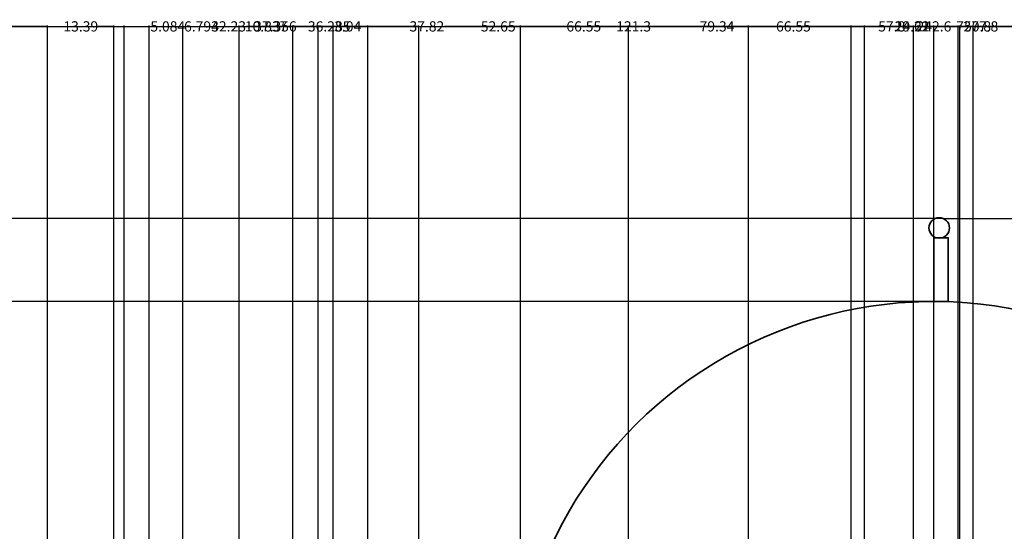
# Model space of a CAD drawing. Units: inches. Extents: x 14 to 859, y 52 to 711.
# Tile 8 of 11: x 244 to 442, y 608 to 711. Entities that reach past the tile are written whole.
import ezdxf

# ---------------------------------------------------------------- set-up
doc = ezdxf.new("R2010")
doc.units = ezdxf.units.IN
doc.header["$MEASUREMENT"] = 0
doc.layers.add('A-ANNO-DIMS', color=2, linetype='Continuous', lineweight=18)
doc.layers.add('A-ROOF', color=7, linetype='Continuous', lineweight=35)
doc.styles.get("Standard").update_dxf_attribs({"font": 'arial.ttf'})
doc.dimstyles.get("Standard").update_dxf_attribs({"dimtxt": 2.0625, "dimasz": 0.18, "dimexe": 0.18, "dimexo": 0.0625, "dimgap": 0.09, "dimtad": 0, "dimtih": 1, "dimtoh": 1, "dimdec": 4, "dimzin": 0, "dimdsep": 46, "dimlunit": 4, "dimtxsty": 'Standard', "dimcen": 0.09, "dimadec": 0, "dimazin": 0, "dimtfac": 1, "dimtdec": 4, "dimtofl": 0, "dimtmove": 0, "dimatfit": 3, "dimfxl": 1, "dimtolj": 1, "dimtzin": 0, "dimarcsym": 0})

# ---------------------------------------------------------------- blocks, each defined once
blk = doc.blocks.new('*D13')
at = {"layer": 'A-ANNO-DIMS', "color": 0, "lineweight": -2, "transparency": 16777216}
for p, q in [((60.78, 339.73), (60.78, 709.71)), ((811.55, 339.73), (811.55, 709.71)), ((60.96, 709.53), (432.6, 709.53)), ((811.37, 709.53), (439.73, 709.53))]:
    blk.add_line(p, q, dxfattribs=at)
at = {"layer": 'A-ANNO-DIMS', "color": 0, "transparency": 16777216}
for points in [[(60.96, 709.56), (60.96, 709.5), (60.78, 709.53)], [(811.37, 709.56), (811.37, 709.5), (811.55, 709.53)]]:
    blk.add_solid(points, dxfattribs=at)
at = {"layer": 'Defpoints', "color": 0, "transparency": 16777216}
for p in [(811.55, 709.53), (60.78, 339.66), (811.55, 339.66)]:
    blk.add_point(p, dxfattribs=at)
at = {"layer": 'A-ANNO-DIMS', "color": 0, "transparency": 16777216, "insert": (436.17, 709.53), "char_height": 2.062, "attachment_point": 5}
blk.add_mtext('\\A1;750.8', dxfattribs=at)
blk = doc.blocks.new('*D16')
at = {"layer": 'A-ANNO-DIMS', "color": 0, "lineweight": -2, "transparency": 16777216}
for p, q in [((429.96, 670.76), (17.7, 670.76)), ((17.88, 670.58), (17.88, 384.41)), ((17.88, 95.97), (17.88, 382.14)), ((60.72, 95.79), (17.7, 95.79))]:
    blk.add_line(p, q, dxfattribs=at)
at = {"layer": 'A-ANNO-DIMS', "color": 0, "transparency": 16777216}
for points in [[(17.85, 670.58), (17.91, 670.58), (17.88, 670.76)], [(17.85, 95.97), (17.91, 95.97), (17.88, 95.79)]]:
    blk.add_solid(points, dxfattribs=at)
at = {"layer": 'Defpoints', "color": 0, "transparency": 16777216}
for p in [(17.88, 670.76), (430.02, 670.76), (60.78, 95.79)]:
    blk.add_point(p, dxfattribs=at)
at = {"layer": 'A-ANNO-DIMS', "color": 0, "transparency": 16777216, "insert": (17.88, 383.28), "char_height": 2.062, "attachment_point": 5}
blk.add_mtext('\\A1;575', dxfattribs=at)
blk = doc.blocks.new('*D19')
at = {"layer": 'A-ANNO-DIMS', "color": 0, "lineweight": -2, "transparency": 16777216}
for p, q in [((430.09, 670.76), (854.64, 670.76)), ((854.46, 670.58), (854.46, 538.71)), ((854.46, 404.55), (854.46, 536.42)), ((609.81, 404.37), (854.64, 404.37))]:
    blk.add_line(p, q, dxfattribs=at)
at = {"layer": 'A-ANNO-DIMS', "color": 0, "transparency": 16777216}
for points in [[(854.43, 670.58), (854.49, 670.58), (854.46, 670.76)], [(854.43, 404.55), (854.49, 404.55), (854.46, 404.37)]]:
    blk.add_solid(points, dxfattribs=at)
at = {"layer": 'Defpoints', "color": 0, "transparency": 16777216}
for p in [(430.02, 670.76), (854.46, 670.76), (609.75, 404.37)]:
    blk.add_point(p, dxfattribs=at)
at = {"layer": 'A-ANNO-DIMS', "color": 0, "transparency": 16777216, "insert": (854.46, 537.57), "char_height": 2.062, "attachment_point": 5}
blk.add_mtext('\\A1;266.4', dxfattribs=at)
blk = doc.blocks.new('*D21')
at = {"layer": 'A-ANNO-DIMS', "color": 0, "lineweight": -2, "transparency": 16777216}
for p, q in [((287.89, 352.49), (287.89, 709.71)), ((298.73, 341.73), (298.73, 709.71)), ((288.07, 709.53), (289.04, 709.53)), ((298.55, 709.53), (297.59, 709.53))]:
    blk.add_line(p, q, dxfattribs=at)
at = {"layer": 'A-ANNO-DIMS', "color": 0, "transparency": 16777216}
for points in [[(288.07, 709.56), (288.07, 709.5), (287.89, 709.53)], [(298.55, 709.56), (298.55, 709.5), (298.73, 709.53)]]:
    blk.add_solid(points, dxfattribs=at)
at = {"layer": 'Defpoints', "color": 0, "transparency": 16777216}
for p in [(298.73, 709.53), (287.89, 352.43), (298.73, 341.67)]:
    blk.add_point(p, dxfattribs=at)
at = {"layer": 'A-ANNO-DIMS', "color": 0, "transparency": 16777216, "insert": (293.31, 709.53), "char_height": 2.062, "attachment_point": 5}
blk.add_mtext('\\A1;10.837', dxfattribs=at)
blk = doc.blocks.new('*D22')
at = {"layer": 'A-ANNO-DIMS', "color": 0, "lineweight": -2, "transparency": 16777216}
for p, q in [((298.73, 341.73), (298.73, 709.71)), ((576.51, 341.73), (576.51, 709.71)), ((298.91, 709.53), (434.03, 709.53)), ((576.33, 709.53), (441.21, 709.53))]:
    blk.add_line(p, q, dxfattribs=at)
at = {"layer": 'A-ANNO-DIMS', "color": 0, "transparency": 16777216}
for points in [[(298.91, 709.56), (298.91, 709.5), (298.73, 709.53)], [(576.33, 709.56), (576.33, 709.5), (576.51, 709.53)]]:
    blk.add_solid(points, dxfattribs=at)
at = {"layer": 'Defpoints', "color": 0, "transparency": 16777216}
for p in [(576.51, 709.53), (298.73, 341.67), (576.51, 341.67)]:
    blk.add_point(p, dxfattribs=at)
at = {"layer": 'A-ANNO-DIMS', "color": 0, "transparency": 16777216, "insert": (437.62, 709.53), "char_height": 2.062, "attachment_point": 5}
blk.add_mtext('\\A1;277.8', dxfattribs=at)
blk = doc.blocks.new('*D66')
at = {"layer": 'A-ANNO-DIMS', "color": 0, "lineweight": -2, "transparency": 16777216}
for p, q in [((223.53, 404.43), (223.53, 709.71)), ((249.19, 404.43), (249.19, 709.71)), ((223.71, 709.53), (232.77, 709.53)), ((249.01, 709.53), (239.95, 709.53))]:
    blk.add_line(p, q, dxfattribs=at)
at = {"layer": 'A-ANNO-DIMS', "color": 0, "transparency": 16777216}
for points in [[(223.71, 709.56), (223.71, 709.5), (223.53, 709.53)], [(249.01, 709.56), (249.01, 709.5), (249.19, 709.53)]]:
    blk.add_solid(points, dxfattribs=at)
at = {"layer": 'Defpoints', "color": 0, "transparency": 16777216}
for p in [(249.19, 709.53), (223.53, 404.37), (249.19, 404.37)]:
    blk.add_point(p, dxfattribs=at)
at = {"layer": 'A-ANNO-DIMS', "color": 0, "transparency": 16777216, "insert": (236.36, 709.53), "char_height": 2.062, "attachment_point": 5}
blk.add_mtext('\\A1;25.67', dxfattribs=at)
blk = doc.blocks.new('*D67')
at = {"layer": 'A-ANNO-DIMS', "color": 0, "lineweight": -2, "transparency": 16777216}
for p, q in [((249.19, 404.43), (249.19, 709.71)), ((262.58, 404.43), (262.58, 709.71)), ((249.37, 709.53), (252.41, 709.53)), ((262.4, 709.53), (259.36, 709.53))]:
    blk.add_line(p, q, dxfattribs=at)
at = {"layer": 'A-ANNO-DIMS', "color": 0, "transparency": 16777216}
for points in [[(249.37, 709.56), (249.37, 709.5), (249.19, 709.53)], [(262.4, 709.56), (262.4, 709.5), (262.58, 709.53)]]:
    blk.add_solid(points, dxfattribs=at)
at = {"layer": 'Defpoints', "color": 0, "transparency": 16777216}
for p in [(262.58, 709.53), (249.19, 404.37), (262.58, 404.37)]:
    blk.add_point(p, dxfattribs=at)
at = {"layer": 'A-ANNO-DIMS', "color": 0, "transparency": 16777216, "insert": (255.89, 709.53), "char_height": 2.062, "attachment_point": 5}
blk.add_mtext('\\A1;13.39', dxfattribs=at)
blk = doc.blocks.new('*D93')
at = {"layer": 'A-ANNO-DIMS', "color": 0, "lineweight": -2, "transparency": 16777216}
for p, q in [((429.22, 654.01), (17.7, 654.01)), ((17.88, 653.83), (17.88, 612.51)), ((17.88, 568.92), (17.88, 610.23)), ((342.81, 568.74), (17.7, 568.74))]:
    blk.add_line(p, q, dxfattribs=at)
at = {"layer": 'A-ANNO-DIMS', "color": 0, "transparency": 16777216}
for points in [[(17.85, 653.83), (17.91, 653.83), (17.88, 654.01)], [(17.85, 568.92), (17.91, 568.92), (17.88, 568.74)]]:
    blk.add_solid(points, dxfattribs=at)
at = {"layer": 'Defpoints', "color": 0, "transparency": 16777216}
for p in [(17.88, 654.01), (429.29, 654.01), (342.87, 568.74)]:
    blk.add_point(p, dxfattribs=at)
at = {"layer": 'A-ANNO-DIMS', "color": 0, "transparency": 16777216, "insert": (17.88, 611.37), "char_height": 2.062, "attachment_point": 5}
blk.add_mtext('\\A1;85.27', dxfattribs=at)
blk = doc.blocks.new('*D94')
at = {"layer": 'A-ANNO-DIMS', "color": 0, "lineweight": -2, "transparency": 16777216}
for p, q in [((429.96, 670.76), (17.7, 670.76)), ((17.88, 670.58), (17.88, 663.53)), ((17.88, 654.19), (17.88, 661.24)), ((429.22, 654.01), (17.7, 654.01))]:
    blk.add_line(p, q, dxfattribs=at)
at = {"layer": 'A-ANNO-DIMS', "color": 0, "transparency": 16777216}
for points in [[(17.85, 670.58), (17.91, 670.58), (17.88, 670.76)], [(17.85, 654.19), (17.91, 654.19), (17.88, 654.01)]]:
    blk.add_solid(points, dxfattribs=at)
at = {"layer": 'Defpoints', "color": 0, "transparency": 16777216}
for p in [(17.88, 670.76), (430.02, 670.76), (429.29, 654.01)]:
    blk.add_point(p, dxfattribs=at)
at = {"layer": 'A-ANNO-DIMS', "color": 0, "transparency": 16777216, "insert": (17.88, 662.38), "char_height": 2.062, "attachment_point": 5}
blk.add_mtext('\\A1;16.758', dxfattribs=at)
blk = doc.blocks.new('*D95')
at = {"layer": 'A-ANNO-DIMS', "color": 0, "lineweight": -2, "transparency": 16777216}
for p, q in [((276.5, 504.44), (276.5, 709.71)), ((313.86, 504.44), (313.86, 709.71)), ((276.68, 709.53), (290.81, 709.53)), ((313.68, 709.53), (299.55, 709.53))]:
    blk.add_line(p, q, dxfattribs=at)
at = {"layer": 'A-ANNO-DIMS', "color": 0, "transparency": 16777216}
for points in [[(276.68, 709.56), (276.68, 709.5), (276.5, 709.53)], [(313.68, 709.56), (313.68, 709.5), (313.86, 709.53)]]:
    blk.add_solid(points, dxfattribs=at)
at = {"layer": 'Defpoints', "color": 0, "transparency": 16777216}
for p in [(313.86, 709.53), (276.5, 504.38), (313.86, 504.38)]:
    blk.add_point(p, dxfattribs=at)
at = {"layer": 'A-ANNO-DIMS', "color": 0, "transparency": 16777216, "insert": (295.18, 709.53), "char_height": 2.062, "attachment_point": 5}
blk.add_mtext('\\A1;37.356', dxfattribs=at)
blk = doc.blocks.new('*D96')
at = {"layer": 'A-ANNO-DIMS', "color": 0, "lineweight": -2, "transparency": 16777216}
for p, q in [((313.86, 504.44), (313.86, 709.71)), ((366.51, 447.01), (366.51, 709.71)), ((314.04, 709.53), (336.61, 709.53)), ((366.33, 709.53), (343.76, 709.53))]:
    blk.add_line(p, q, dxfattribs=at)
at = {"layer": 'A-ANNO-DIMS', "color": 0, "transparency": 16777216}
for points in [[(314.04, 709.56), (314.04, 709.5), (313.86, 709.53)], [(366.33, 709.56), (366.33, 709.5), (366.51, 709.53)]]:
    blk.add_solid(points, dxfattribs=at)
at = {"layer": 'Defpoints', "color": 0, "transparency": 16777216}
for p in [(366.51, 709.53), (313.86, 504.38), (366.51, 446.95)]:
    blk.add_point(p, dxfattribs=at)
at = {"layer": 'A-ANNO-DIMS', "color": 0, "transparency": 16777216, "insert": (340.18, 709.53), "char_height": 2.062, "attachment_point": 5}
blk.add_mtext('\\A1;52.65', dxfattribs=at)
blk = doc.blocks.new('*D97')
at = {"layer": 'A-ANNO-DIMS', "color": 0, "lineweight": -2, "transparency": 16777216}
for p, q in [((366.51, 447.01), (366.51, 709.71)), ((433.06, 447.01), (433.06, 709.71)), ((366.69, 709.53), (396.2, 709.53)), ((432.88, 709.53), (403.37, 709.53))]:
    blk.add_line(p, q, dxfattribs=at)
at = {"layer": 'A-ANNO-DIMS', "color": 0, "transparency": 16777216}
for points in [[(366.69, 709.56), (366.69, 709.5), (366.51, 709.53)], [(432.88, 709.56), (432.88, 709.5), (433.06, 709.53)]]:
    blk.add_solid(points, dxfattribs=at)
at = {"layer": 'Defpoints', "color": 0, "transparency": 16777216}
for p in [(433.06, 709.53), (366.51, 446.95), (433.06, 446.95)]:
    blk.add_point(p, dxfattribs=at)
at = {"layer": 'A-ANNO-DIMS', "color": 0, "transparency": 16777216, "insert": (399.78, 709.53), "char_height": 2.062, "attachment_point": 5}
blk.add_mtext('\\A1;66.55', dxfattribs=at)
blk = doc.blocks.new('*D98')
at = {"layer": 'A-ANNO-DIMS', "color": 0, "lineweight": -2, "transparency": 16777216}
for p, q in [((433.06, 447.01), (433.06, 709.71)), ((505.25, 447.01), (505.25, 709.71)), ((433.24, 709.53), (465.59, 709.53)), ((505.07, 709.53), (472.72, 709.53))]:
    blk.add_line(p, q, dxfattribs=at)
at = {"layer": 'A-ANNO-DIMS', "color": 0, "transparency": 16777216}
for points in [[(433.24, 709.56), (433.24, 709.5), (433.06, 709.53)], [(505.07, 709.56), (505.07, 709.5), (505.25, 709.53)]]:
    blk.add_solid(points, dxfattribs=at)
at = {"layer": 'Defpoints', "color": 0, "transparency": 16777216}
for p in [(505.25, 709.53), (433.06, 446.95), (505.25, 446.95)]:
    blk.add_point(p, dxfattribs=at)
at = {"layer": 'A-ANNO-DIMS', "color": 0, "transparency": 16777216, "insert": (469.15, 709.53), "char_height": 2.062, "attachment_point": 5}
blk.add_mtext('\\A1;72.19', dxfattribs=at)
blk = doc.blocks.new('*D104')
at = {"layer": 'A-ANNO-DIMS', "color": 0, "lineweight": -2, "transparency": 16777216}
for p, q in [((264.63, 519.11), (264.63, 709.71)), ((269.71, 515.26), (269.71, 709.71)), ((264.81, 709.53), (269.53, 709.53)), ((269.71, 709.53), (269.89, 709.53))]:
    blk.add_line(p, q, dxfattribs=at)
at = {"layer": 'A-ANNO-DIMS', "color": 0, "transparency": 16777216}
for points in [[(264.81, 709.56), (264.81, 709.5), (264.63, 709.53)], [(269.53, 709.56), (269.53, 709.5), (269.71, 709.53)]]:
    blk.add_solid(points, dxfattribs=at)
at = {"layer": 'Defpoints', "color": 0, "transparency": 16777216}
for p in [(269.71, 709.53), (264.63, 519.05), (269.71, 515.2)]:
    blk.add_point(p, dxfattribs=at)
at = {"layer": 'A-ANNO-DIMS', "color": 0, "transparency": 16777216, "insert": (273.46, 709.53), "char_height": 2.062, "attachment_point": 5}
blk.add_mtext('\\A1;5.084', dxfattribs=at)
blk = doc.blocks.new('*D105')
at = {"layer": 'A-ANNO-DIMS', "color": 0, "lineweight": -2, "transparency": 16777216}
for p, q in [((306.86, 560.74), (306.86, 709.71)), ((549.44, 560.74), (549.44, 709.71)), ((307.04, 709.53), (424.56, 709.53)), ((549.26, 709.53), (431.74, 709.53))]:
    blk.add_line(p, q, dxfattribs=at)
at = {"layer": 'A-ANNO-DIMS', "color": 0, "transparency": 16777216}
for points in [[(307.04, 709.56), (307.04, 709.5), (306.86, 709.53)], [(549.26, 709.56), (549.26, 709.5), (549.44, 709.53)]]:
    blk.add_solid(points, dxfattribs=at)
at = {"layer": 'Defpoints', "color": 0, "transparency": 16777216}
for p in [(549.44, 709.53), (306.86, 560.68), (549.44, 560.68)]:
    blk.add_point(p, dxfattribs=at)
at = {"layer": 'A-ANNO-DIMS', "color": 0, "transparency": 16777216, "insert": (428.15, 709.53), "char_height": 2.062, "attachment_point": 5}
blk.add_mtext('\\A1;242.6', dxfattribs=at)
blk = doc.blocks.new('*D106')
at = {"layer": 'A-ANNO-DIMS', "color": 0, "lineweight": -2, "transparency": 16777216}
for p, q in [((303.82, 562.72), (303.82, 709.71)), ((306.86, 560.74), (306.86, 709.71)), ((304, 709.53), (306.68, 709.53)), ((306.86, 709.53), (307.04, 709.53))]:
    blk.add_line(p, q, dxfattribs=at)
at = {"layer": 'A-ANNO-DIMS', "color": 0, "transparency": 16777216}
for points in [[(304, 709.56), (304, 709.5), (303.82, 709.53)], [(306.68, 709.56), (306.68, 709.5), (306.86, 709.53)]]:
    blk.add_solid(points, dxfattribs=at)
at = {"layer": 'Defpoints', "color": 0, "transparency": 16777216}
for p in [(306.86, 709.53), (303.82, 562.66), (306.86, 560.68)]:
    blk.add_point(p, dxfattribs=at)
at = {"layer": 'A-ANNO-DIMS', "color": 0, "transparency": 16777216, "insert": (309.8, 709.53), "char_height": 2.062, "attachment_point": 5}
blk.add_mtext('\\A1;3.04', dxfattribs=at)
blk = doc.blocks.new('*D108')
at = {"layer": 'A-ANNO-DIMS', "color": 0, "lineweight": -2, "transparency": 16777216}
for p, q in [((264.63, 519.11), (264.63, 709.71)), ((306.86, 560.74), (306.86, 709.71)), ((264.81, 709.53), (282.13, 709.53)), ((306.68, 709.53), (289.36, 709.53))]:
    blk.add_line(p, q, dxfattribs=at)
at = {"layer": 'A-ANNO-DIMS', "color": 0, "transparency": 16777216}
for points in [[(264.81, 709.56), (264.81, 709.5), (264.63, 709.53)], [(306.68, 709.56), (306.68, 709.5), (306.86, 709.53)]]:
    blk.add_solid(points, dxfattribs=at)
at = {"layer": 'Defpoints', "color": 0, "transparency": 16777216}
for p in [(306.86, 709.53), (306.86, 560.68), (264.63, 519.05)]:
    blk.add_point(p, dxfattribs=at)
at = {"layer": 'A-ANNO-DIMS', "color": 0, "transparency": 16777216, "insert": (285.74, 709.53), "char_height": 2.062, "attachment_point": 5}
blk.add_mtext('\\A1;42.23', dxfattribs=at)
blk = doc.blocks.new('*D109')
at = {"layer": 'A-ANNO-DIMS', "color": 0, "lineweight": -2, "transparency": 16777216}
for p, q in [((269.71, 515.26), (269.71, 709.71)), ((276.5, 509.85), (276.5, 709.71)), ((269.89, 709.53), (276.32, 709.53)), ((276.5, 709.53), (276.68, 709.53))]:
    blk.add_line(p, q, dxfattribs=at)
at = {"layer": 'A-ANNO-DIMS', "color": 0, "transparency": 16777216}
for points in [[(269.89, 709.56), (269.89, 709.5), (269.71, 709.53)], [(276.32, 709.56), (276.32, 709.5), (276.5, 709.53)]]:
    blk.add_solid(points, dxfattribs=at)
at = {"layer": 'Defpoints', "color": 0, "transparency": 16777216}
for p in [(276.5, 709.53), (269.71, 515.2), (276.5, 509.79)]:
    blk.add_point(p, dxfattribs=at)
at = {"layer": 'A-ANNO-DIMS', "color": 0, "transparency": 16777216, "insert": (280.26, 709.53), "char_height": 2.062, "attachment_point": 5}
blk.add_mtext('\\A1;6.793', dxfattribs=at)
blk = doc.blocks.new('*D110')
at = {"layer": 'A-ANNO-DIMS', "color": 0, "lineweight": -2, "transparency": 16777216}
for p, q in [((306.86, 518.73), (306.86, 709.71)), ((344.68, 539), (344.68, 709.71)), ((307.04, 709.53), (322.21, 709.53)), ((344.5, 709.53), (329.33, 709.53))]:
    blk.add_line(p, q, dxfattribs=at)
at = {"layer": 'A-ANNO-DIMS', "color": 0, "transparency": 16777216}
for points in [[(307.04, 709.56), (307.04, 709.5), (306.86, 709.53)], [(344.5, 709.56), (344.5, 709.5), (344.68, 709.53)]]:
    blk.add_solid(points, dxfattribs=at)
at = {"layer": 'Defpoints', "color": 0, "transparency": 16777216}
for p in [(344.68, 709.53), (344.68, 538.94), (306.86, 518.67)]:
    blk.add_point(p, dxfattribs=at)
at = {"layer": 'A-ANNO-DIMS', "color": 0, "transparency": 16777216, "insert": (325.77, 709.53), "char_height": 2.062, "attachment_point": 5}
blk.add_mtext('\\A1;37.82', dxfattribs=at)
blk = doc.blocks.new('*D111')
at = {"layer": 'A-ANNO-DIMS', "color": 0, "lineweight": -2, "transparency": 16777216}
for p, q in [((344.68, 539), (344.68, 709.71)), ((424.02, 539), (424.02, 709.71)), ((344.86, 709.53), (380.79, 709.53)), ((423.84, 709.53), (387.91, 709.53))]:
    blk.add_line(p, q, dxfattribs=at)
at = {"layer": 'A-ANNO-DIMS', "color": 0, "transparency": 16777216}
for points in [[(344.86, 709.56), (344.86, 709.5), (344.68, 709.53)], [(423.84, 709.56), (423.84, 709.5), (424.02, 709.53)]]:
    blk.add_solid(points, dxfattribs=at)
at = {"layer": 'Defpoints', "color": 0, "transparency": 16777216}
for p in [(424.02, 709.53), (344.68, 538.94), (424.02, 538.94)]:
    blk.add_point(p, dxfattribs=at)
at = {"layer": 'A-ANNO-DIMS', "color": 0, "transparency": 16777216, "insert": (384.35, 709.53), "char_height": 2.062, "attachment_point": 5}
blk.add_mtext('\\A1;79.34', dxfattribs=at)
blk = doc.blocks.new('*D112')
at = {"layer": 'A-ANNO-DIMS', "color": 0, "lineweight": -2, "transparency": 16777216}
for p, q in [((424.02, 539), (424.02, 709.71)), ((508.63, 539), (508.63, 709.71)), ((424.2, 709.53), (462.95, 709.53)), ((508.45, 709.53), (469.7, 709.53))]:
    blk.add_line(p, q, dxfattribs=at)
at = {"layer": 'A-ANNO-DIMS', "color": 0, "transparency": 16777216}
for points in [[(424.2, 709.56), (424.2, 709.5), (424.02, 709.53)], [(508.45, 709.56), (508.45, 709.5), (508.63, 709.53)]]:
    blk.add_solid(points, dxfattribs=at)
at = {"layer": 'Defpoints', "color": 0, "transparency": 16777216}
for p in [(508.63, 709.53), (424.02, 538.94), (508.63, 538.94)]:
    blk.add_point(p, dxfattribs=at)
at = {"layer": 'A-ANNO-DIMS', "color": 0, "transparency": 16777216, "insert": (466.32, 709.53), "char_height": 2.062, "attachment_point": 5}
blk.add_mtext('\\A1;84.61', dxfattribs=at)
blk = doc.blocks.new('*D114')
at = {"layer": 'A-ANNO-DIMS', "color": 0, "lineweight": -2, "transparency": 16777216}
for p, q in [((411.43, 534.21), (411.43, 709.71)), ((436.05, 534.21), (436.05, 709.71)), ((411.61, 709.53), (420.17, 709.53)), ((435.87, 709.53), (427.32, 709.53))]:
    blk.add_line(p, q, dxfattribs=at)
at = {"layer": 'A-ANNO-DIMS', "color": 0, "transparency": 16777216}
for points in [[(411.61, 709.56), (411.61, 709.5), (411.43, 709.53)], [(435.87, 709.56), (435.87, 709.5), (436.05, 709.53)]]:
    blk.add_solid(points, dxfattribs=at)
at = {"layer": 'Defpoints', "color": 0, "transparency": 16777216}
for p in [(436.05, 709.53), (411.43, 534.15), (436.05, 534.15)]:
    blk.add_point(p, dxfattribs=at)
at = {"layer": 'A-ANNO-DIMS', "color": 0, "transparency": 16777216, "insert": (423.74, 709.53), "char_height": 2.062, "attachment_point": 5}
blk.add_mtext('\\A1;24.62', dxfattribs=at)
blk = doc.blocks.new('*D115')
at = {"layer": 'A-ANNO-DIMS', "color": 0, "lineweight": -2, "transparency": 16777216}
for p, q in [((414.14, 531.51), (414.14, 709.71)), ((433.35, 531.51), (433.35, 709.71)), ((414.32, 709.53), (420.47, 709.53)), ((433.17, 709.53), (427.02, 709.53))]:
    blk.add_line(p, q, dxfattribs=at)
at = {"layer": 'A-ANNO-DIMS', "color": 0, "transparency": 16777216}
for points in [[(414.32, 709.56), (414.32, 709.5), (414.14, 709.53)], [(433.17, 709.56), (433.17, 709.5), (433.35, 709.53)]]:
    blk.add_solid(points, dxfattribs=at)
at = {"layer": 'Defpoints', "color": 0, "transparency": 16777216}
for p in [(433.35, 709.53), (414.14, 531.45), (433.35, 531.45)]:
    blk.add_point(p, dxfattribs=at)
at = {"layer": 'A-ANNO-DIMS', "color": 0, "transparency": 16777216, "insert": (423.74, 709.53), "char_height": 2.062, "attachment_point": 5}
blk.add_mtext('\\A1;19.21', dxfattribs=at)
blk = doc.blocks.new('*D118')
at = {"layer": 'A-ANNO-DIMS', "color": 0, "lineweight": -2, "transparency": 16777216}
for p, q in [((306.86, 560.74), (306.86, 709.71)), ((428.15, 568.8), (428.15, 709.71)), ((307.04, 709.53), (364.03, 709.53)), ((427.97, 709.53), (370.98, 709.53))]:
    blk.add_line(p, q, dxfattribs=at)
at = {"layer": 'A-ANNO-DIMS', "color": 0, "transparency": 16777216}
for points in [[(307.04, 709.56), (307.04, 709.5), (306.86, 709.53)], [(427.97, 709.56), (427.97, 709.5), (428.15, 709.53)]]:
    blk.add_solid(points, dxfattribs=at)
at = {"layer": 'Defpoints', "color": 0, "transparency": 16777216}
for p in [(428.15, 709.53), (428.15, 568.74), (306.86, 560.68)]:
    blk.add_point(p, dxfattribs=at)
at = {"layer": 'A-ANNO-DIMS', "color": 0, "transparency": 16777216, "insert": (367.51, 709.53), "char_height": 2.062, "attachment_point": 5}
blk.add_mtext('\\A1;121.3', dxfattribs=at)
blk = doc.blocks.new('*D119')
at = {"layer": 'A-ANNO-DIMS', "color": 0, "lineweight": -2, "transparency": 16777216}
for p, q in [((287.89, 404.43), (287.89, 709.71)), ((324.18, 404.43), (324.18, 709.71)), ((288.07, 709.53), (301.66, 709.53)), ((324, 709.53), (310.41, 709.53))]:
    blk.add_line(p, q, dxfattribs=at)
at = {"layer": 'A-ANNO-DIMS', "color": 0, "transparency": 16777216}
for points in [[(288.07, 709.56), (288.07, 709.5), (287.89, 709.53)], [(324, 709.56), (324, 709.5), (324.18, 709.53)]]:
    blk.add_solid(points, dxfattribs=at)
at = {"layer": 'Defpoints', "color": 0, "transparency": 16777216}
for p in [(324.18, 709.53), (287.89, 404.37), (324.18, 404.37)]:
    blk.add_point(p, dxfattribs=at)
at = {"layer": 'A-ANNO-DIMS', "color": 0, "transparency": 16777216, "insert": (306.04, 709.53), "char_height": 2.062, "attachment_point": 5}
blk.add_mtext('\\A1;36.285', dxfattribs=at)
blk = doc.blocks.new('*D120')
at = {"layer": 'A-ANNO-DIMS', "color": 0, "lineweight": -2, "transparency": 16777216}
for p, q in [((324.18, 404.43), (324.18, 709.71)), ((390.73, 404.43), (390.73, 709.71)), ((324.36, 709.53), (353.87, 709.53)), ((390.55, 709.53), (361.04, 709.53))]:
    blk.add_line(p, q, dxfattribs=at)
at = {"layer": 'A-ANNO-DIMS', "color": 0, "transparency": 16777216}
for points in [[(324.36, 709.56), (324.36, 709.5), (324.18, 709.53)], [(390.55, 709.56), (390.55, 709.5), (390.73, 709.53)]]:
    blk.add_solid(points, dxfattribs=at)
at = {"layer": 'Defpoints', "color": 0, "transparency": 16777216}
for p in [(390.73, 709.53), (324.18, 404.37), (390.73, 404.37)]:
    blk.add_point(p, dxfattribs=at)
at = {"layer": 'A-ANNO-DIMS', "color": 0, "transparency": 16777216, "insert": (357.45, 709.53), "char_height": 2.062, "attachment_point": 5}
blk.add_mtext('\\A1;66.55', dxfattribs=at)
blk = doc.blocks.new('*D121')
at = {"layer": 'A-ANNO-DIMS', "color": 0, "lineweight": -2, "transparency": 16777216}
for p, q in [((390.73, 404.43), (390.73, 709.71)), ((448.54, 404.43), (448.54, 709.71)), ((390.91, 709.53), (416.86, 709.53)), ((448.36, 709.53), (422.4, 709.53))]:
    blk.add_line(p, q, dxfattribs=at)
at = {"layer": 'A-ANNO-DIMS', "color": 0, "transparency": 16777216}
for points in [[(390.91, 709.56), (390.91, 709.5), (390.73, 709.53)], [(448.36, 709.56), (448.36, 709.5), (448.54, 709.53)]]:
    blk.add_solid(points, dxfattribs=at)
at = {"layer": 'Defpoints', "color": 0, "transparency": 16777216}
for p in [(448.54, 709.53), (390.73, 404.37), (448.54, 404.37)]:
    blk.add_point(p, dxfattribs=at)
at = {"layer": 'A-ANNO-DIMS', "color": 0, "transparency": 16777216, "insert": (419.63, 709.53), "char_height": 2.062, "attachment_point": 5}
blk.add_mtext('\\A1;57.8', dxfattribs=at)
blk = doc.blocks.new('*D130')
at = {"layer": 'A-ANNO-DIMS', "color": 0, "lineweight": -2, "transparency": 16777216}
for p, q in [((541.65, 644.46), (499.24, 616.16)), ((541.83, 644.46), (541.65, 644.46)), ((428.06, 568.74), (428.24, 568.74)), ((428.15, 568.65), (428.15, 568.83))]:
    blk.add_line(p, q, dxfattribs=at)
at = {"layer": 'A-ANNO-DIMS', "color": 0, "transparency": 16777216}
blk.add_solid([(499.22, 616.19), (499.26, 616.14), (499.09, 616.06)], dxfattribs=at)
at = {"layer": 'Defpoints', "color": 0, "transparency": 16777216}
for p in [(499.09, 616.06), (428.15, 568.74)]:
    blk.add_point(p, dxfattribs=at)
at = {"layer": 'A-ANNO-DIMS', "color": 0, "transparency": 16777216, "insert": (546.39, 644.46), "char_height": 2.062, "attachment_point": 5}
blk.add_mtext('\\A1;R85.28', dxfattribs=at)

msp = doc.modelspace()

# ---------------------------------------------------------------- linework, layer by layer
at = {"layer": 'A-ROOF'}
msp.add_lwpolyline([(428.1517, 654.0137), (431.0349, 654.0137), (431.0349, 666.8234), (428.1517, 666.8234)], close=True, dxfattribs=at)
msp.add_circle((429.2176, 668.8576), 2.0686, dxfattribs=at)
msp.add_arc((428.1517, 568.7358), 85.2778, 358.475544, 180, dxfattribs=at)

# ---------------------------------------------------------------- dimensions: what is measured, and where the dimension line sits
at = {"layer": 'A-ANNO-DIMS'}
for base, p1, p2, override, picture, middle in [((811.5534, 709.5262), (60.7804, 339.6626), (811.5534, 339.6626), {"dimdec": 1, "dimlfac": 1, "dimrnd": 0, "dimzin": 0, "dimdsep": 46, "dimlunit": 2}, '*D13', (436.1669, 709.5262)), ((249.1939, 709.5262), (223.5256, 404.3712), (249.1939, 404.3712), {"dimdec": 2, "dimlfac": 1, "dimrnd": 0, "dimzin": 0, "dimdsep": 46, "dimlunit": 2}, '*D66', (236.3598, 709.5262)), ((262.5837, 709.5262), (249.1939, 404.3712), (262.5837, 404.3712), {"dimdec": 2, "dimlfac": 1, "dimrnd": 0, "dimzin": 0, "dimdsep": 46, "dimlunit": 2}, '*D67', (255.8888, 709.5262)), ((269.7112, 709.5262), (264.6274, 519.0512), (269.7112, 515.1991), {"dimdec": 3, "dimlfac": 1, "dimrnd": 0, "dimzin": 0, "dimdsep": 46, "dimlunit": 2}, '*D104', (273.457, 709.5262)), ((306.8606, 709.5262), (264.6274, 519.0512), (306.8606, 560.6808), {"dimdec": 2, "dimlfac": 1, "dimrnd": 0, "dimzin": 0, "dimdsep": 46, "dimlunit": 2}, '*D108', (285.744, 709.5262)), ((276.5038, 709.5262), (269.7112, 515.1991), (276.5038, 509.7903), {"dimdec": 3, "dimlfac": 1, "dimrnd": 0, "dimzin": 0, "dimdsep": 46, "dimlunit": 2}, '*D109', (280.2593, 709.5262)), ((313.8595, 709.5262), (276.5038, 504.3815), (313.8595, 504.3815), {"dimdec": 3, "dimlfac": 1, "dimrnd": 0, "dimzin": 0, "dimdsep": 46, "dimlunit": 2}, '*D95', (295.1816, 709.5262)), ((298.72949, 709.52622), (287.89298, 352.42914), (298.72949, 341.67161), {"dimdec": 3, "dimlfac": 1, "dimrnd": 0, "dimzin": 0, "dimdsep": 46, "dimlunit": 2}, '*D21', (293.31124, 709.52622)), ((324.1777, 709.5262), (287.893, 404.3712), (324.1777, 404.3712), {"dimdec": 3, "dimlfac": 1, "dimrnd": 0, "dimzin": 0, "dimdsep": 46, "dimlunit": 2}, '*D119', (306.0353, 709.5262)), ((576.5058, 709.5262), (298.7295, 341.6716), (576.5058, 341.6716), {"dimdec": 1, "dimlfac": 1, "dimrnd": 0, "dimzin": 0, "dimdsep": 46, "dimlunit": 2}, '*D22', (437.6176, 709.5262)), ((306.8606, 709.5262), (303.8209, 562.6585), (306.8606, 560.6808), {"dimdec": 2, "dimlfac": 1, "dimrnd": 0, "dimzin": 0, "dimdsep": 46, "dimlunit": 2}, '*D106', (309.8044, 709.5262)), ((549.4429, 709.5262), (306.8606, 560.6808), (549.4429, 560.6808), {"dimdec": 1, "dimlfac": 1, "dimrnd": 0, "dimzin": 0, "dimdsep": 46, "dimlunit": 2}, '*D105', (428.1517, 709.5262)), ((344.6778, 709.5262), (306.8606, 518.6693), (344.6778, 538.9419), {"dimdec": 2, "dimlfac": 1, "dimrnd": 0, "dimzin": 0, "dimdsep": 46, "dimlunit": 2}, '*D110', (325.7692, 709.5262)), ((428.1517, 709.5262), (306.8606, 560.6808), (428.1517, 568.7358), {"dimdec": 1, "dimlfac": 1, "dimrnd": 0, "dimzin": 0, "dimdsep": 46, "dimlunit": 2}, '*D118', (367.5062, 709.5262)), ((366.507, 709.5262), (313.8595, 504.3815), (366.507, 446.9501), {"dimdec": 2, "dimlfac": 1, "dimrnd": 0, "dimzin": 0, "dimdsep": 46, "dimlunit": 2}, '*D96', (340.1833, 709.5262)), ((390.7307, 709.5262), (324.1777, 404.3712), (390.7307, 404.3712), {"dimdec": 2, "dimlfac": 1, "dimrnd": 0, "dimzin": 0, "dimdsep": 46, "dimlunit": 2}, '*D120', (357.4542, 709.5262)), ((424.0193, 709.5262), (344.6778, 538.9419), (424.0193, 538.9419), {"dimdec": 2, "dimlfac": 1, "dimrnd": 0, "dimzin": 0, "dimdsep": 46, "dimlunit": 2}, '*D111', (384.3486, 709.5262)), ((433.06, 709.5262), (366.507, 446.9501), (433.06, 446.9501), {"dimdec": 2, "dimlfac": 1, "dimrnd": 0, "dimzin": 0, "dimdsep": 46, "dimlunit": 2}, '*D97', (399.7835, 709.5262)), ((448.5359, 709.5262), (390.7307, 404.3712), (448.5359, 404.3712), {"dimdec": 1, "dimlfac": 1, "dimrnd": 0, "dimzin": 0, "dimdsep": 46, "dimlunit": 2}, '*D121', (419.6333, 709.5262)), ((436.0547, 709.5262), (411.435, 534.1509), (436.0547, 534.1509), {"dimdec": 2, "dimlfac": 1, "dimrnd": 0, "dimzin": 0, "dimdsep": 46, "dimlunit": 2}, '*D114', (423.7449, 709.5262)), ((433.3504, 709.5262), (414.1394, 531.4465), (433.3504, 531.4465), {"dimdec": 2, "dimlfac": 1, "dimrnd": 0, "dimzin": 0, "dimdsep": 46, "dimlunit": 2}, '*D115', (423.7449, 709.5262)), ((508.63, 709.5262), (424.0193, 538.9419), (508.63, 538.9419), {"dimdec": 2, "dimlfac": 1, "dimrnd": 0, "dimzin": 0, "dimdsep": 46, "dimlunit": 2}, '*D112', (466.3247, 709.5262)), ((505.2493, 709.5262), (433.06, 446.9501), (505.2493, 446.9501), {"dimdec": 2, "dimlfac": 1, "dimrnd": 0, "dimzin": 0, "dimdsep": 46, "dimlunit": 2}, '*D98', (469.1547, 709.5262))]:
    dim = msp.add_linear_dim(base=base, p1=p1, p2=p2, dimstyle='Standard', override=override, dxfattribs=at)
    dim.commit()
    dim.dimension.update_dxf_attribs({"geometry": picture, "text_midpoint": middle})
for base, p1, p2, override, picture, middle in [((17.8785, 670.7637), (429.2862, 654.0061), (430.0228, 670.7637), {"dimdec": 3, "dimlfac": 1, "dimrnd": 0, "dimzin": 0, "dimdsep": 46, "dimlunit": 2}, '*D94', (17.8785, 662.3849)), ((17.8785, 670.7637), (60.7804, 95.7876), (430.0228, 670.7637), {"dimdec": 0, "dimlfac": 1, "dimrnd": 0, "dimzin": 0, "dimdsep": 46, "dimlunit": 2}, '*D16', (17.8785, 383.2756)), ((854.4554, 670.7637), (609.7501, 404.3712), (430.0228, 670.7637), {"dimdec": 1, "dimlfac": 1, "dimrnd": 0, "dimzin": 0, "dimdsep": 46, "dimlunit": 2}, '*D19', (854.4554, 537.5675)), ((17.8785, 654.0061), (342.8739, 568.7358), (429.2862, 654.0061), {"dimdec": 2, "dimlfac": 1, "dimrnd": 0, "dimzin": 0, "dimdsep": 46, "dimlunit": 2}, '*D93', (17.8785, 611.371))]:
    dim = msp.add_linear_dim(base=base, p1=p1, p2=p2, angle=90, dimstyle='Standard', override=override, dxfattribs=at)
    dim.commit()
    dim.dimension.update_dxf_attribs({"geometry": picture, "text_midpoint": middle})
dim = msp.add_radius_dim(center=(428.1517, 568.7358), mpoint=(499.0902, 616.0649), dimstyle='Standard', override={"dimdec": 2, "dimlfac": 1, "dimrnd": 0, "dimzin": 0, "dimdsep": 46, "dimlunit": 2}, dxfattribs=at)
dim.commit()
dim.dimension.update_dxf_attribs({"geometry": '*D130', "text_midpoint": (546.3923, 644.4623), "dimtype": 164})

doc.saveas('drawing.dxf')
